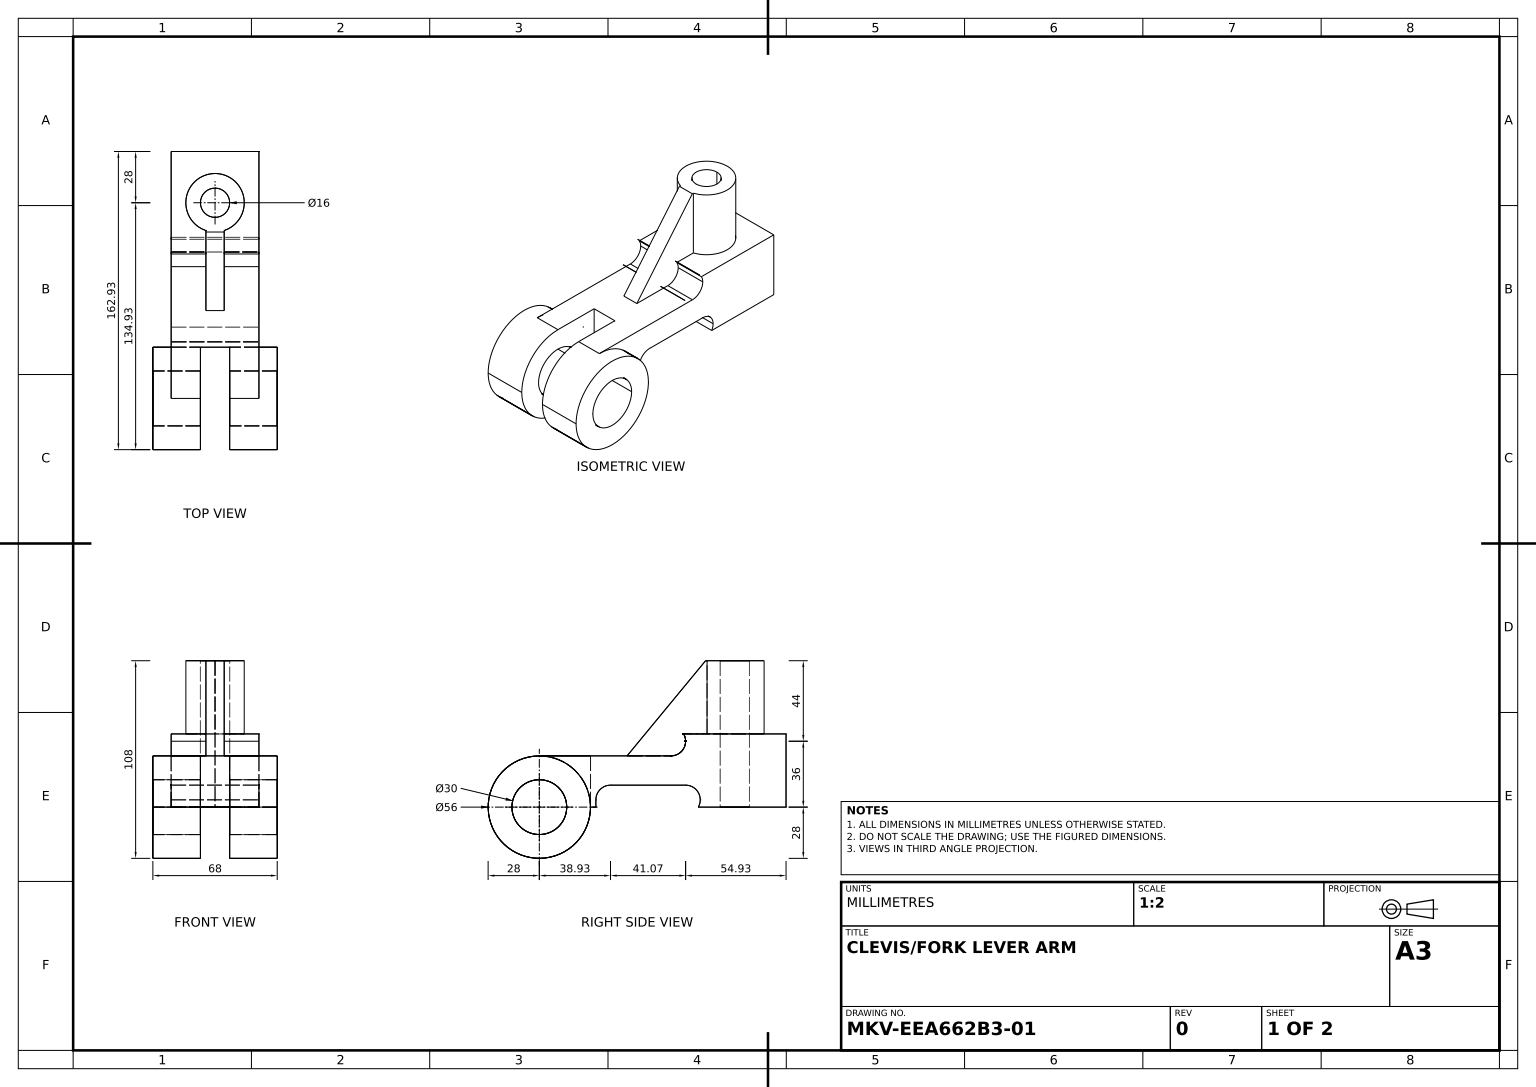
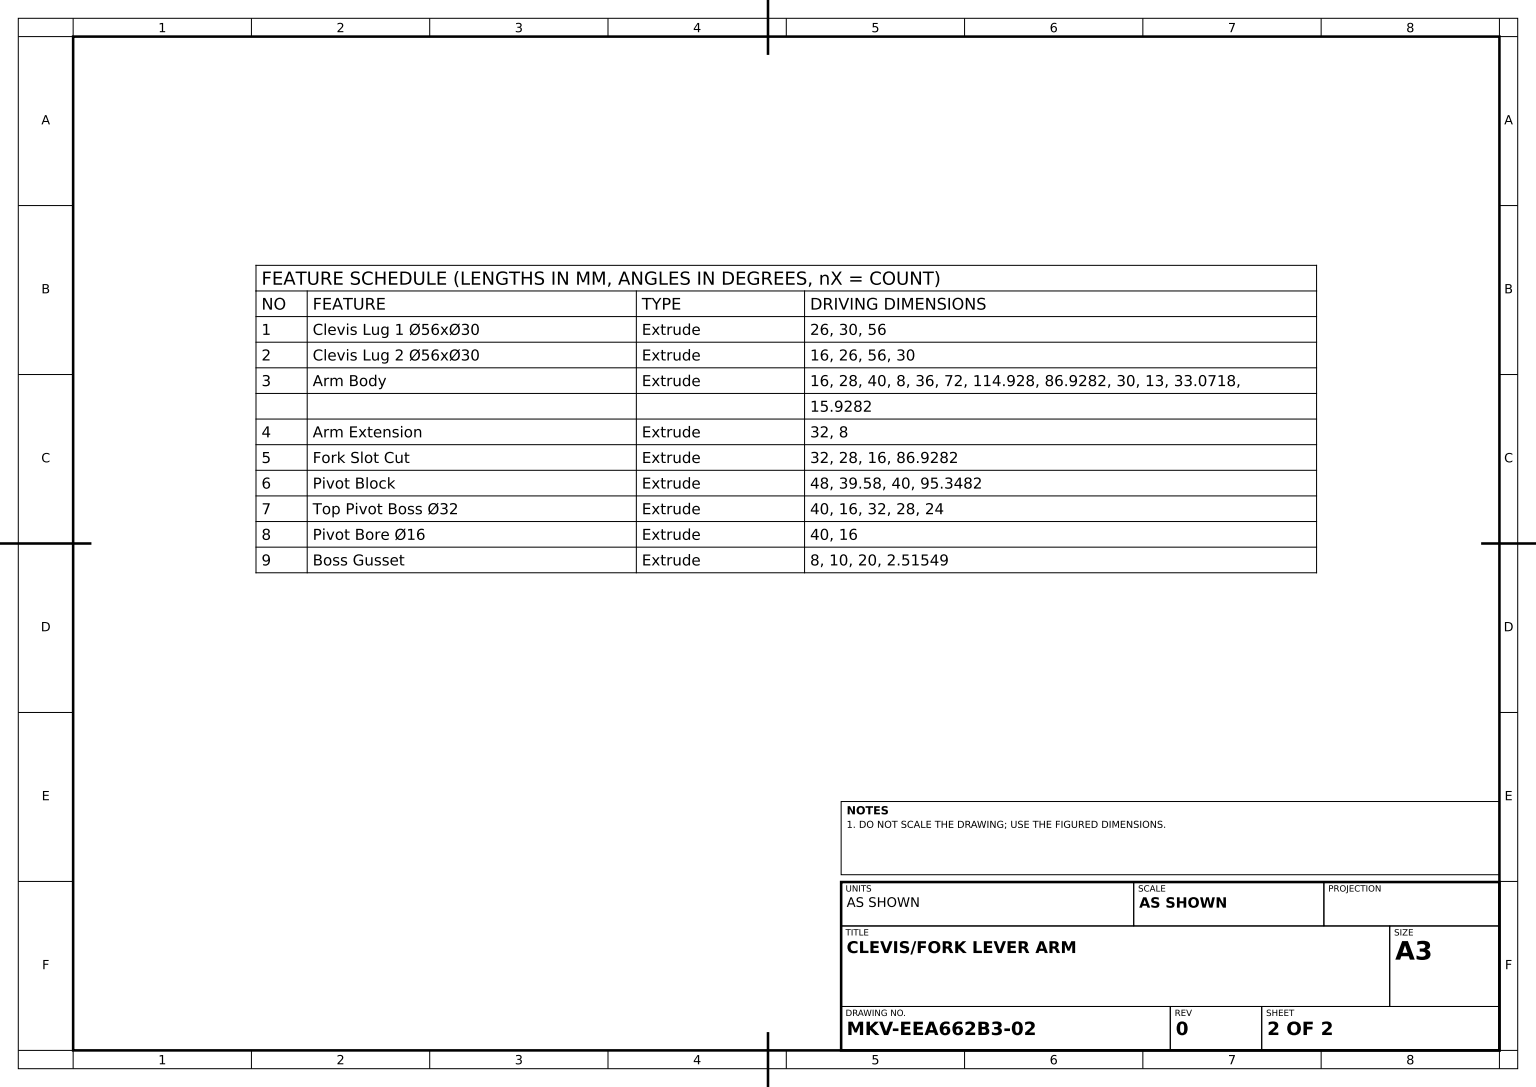
from build123d import *
from build123d.topology import SkipClean

# Parameters (mm, degrees)
CLEVIS_LUG_1_SKETCH_R     = 28
CLEVIS_LUG_1_SKETCH_R_2   = 15
CLEVIS_LUG_1_56X_30_DEPTH = 26
CLEVIS_LUG_2_SKETCH_R     = 28
CLEVIS_LUG_2_SKETCH_R_2   = 15
CLEVIS_LUG_2_56X_30_DEPTH = 26
ARM_START                 = -16
ARM_BODY_DEPTH            = 16
ARM_EXTENSION_DEPTH       = 16
FORK_SLOT_SKETCH_W        = 16
FORK_SLOT_SKETCH_H        = 28
FORK_SLOT_CUT_DEPTH       = 32
PIVOT_BLOCK_SKETCH_W      = 39.579982786
PIVOT_BLOCK_SKETCH_H      = 40
PIVOT_BLOCK_DEPTH         = 48
TOP_PIVOT_BOSS_SKETCH_R   = 16
TOP_PIVOT_BOSS_SKETCH_R_2 = 8
TOP_PIVOT_BOSS_32_DEPTH   = 40
PIVOT_START               = -40
PIVOT_BORE_SKETCH_R       = 8
PIVOT_BORE_16_DEPTH       = 40
BOSS_GUSSET_DEPTH         = 5


with BuildPart() as part:
    # Clevis Lug 1 Sketch → Clevis Lug 1 Ø56xØ30 (new body)
    with BuildSketch(Plane(origin=(0, 0, 0), x_dir=(0, 0, -1), z_dir=(1, 0, 0))):
        with Locations(Location((0, 0, 0), (0, 0, 180))):
            Circle(CLEVIS_LUG_1_SKETCH_R)
        with Locations(Location((0, 0, 0), (0, 0, 180))):
            Circle(CLEVIS_LUG_1_SKETCH_R_2, mode=Mode.SUBTRACT)
    extrude(amount=CLEVIS_LUG_1_56X_30_DEPTH)



with BuildPart() as body_2:
    # Clevis Lug 2 Sketch → Clevis Lug 2 Ø56xØ30 (new body)
    with BuildSketch(Plane(origin=(-16, 0, 0), x_dir=(0, 0, -1), z_dir=(1, 0, 0))):
        with Locations(Location((0, 0, 0), (0, 0, 180))):
            Circle(CLEVIS_LUG_2_SKETCH_R)
        with Locations(Location((0, 0, 0), (0, 0, 180))):
            Circle(CLEVIS_LUG_2_SKETCH_R_2, mode=Mode.SUBTRACT)
    extrude(amount=-CLEVIS_LUG_2_56X_30_DEPTH)

    # Arm Profile Sketch → Arm Body (add)
    with BuildSketch(Plane(origin=(-16, 0, 0), x_dir=(0, 0, -1), z_dir=(1, 0, 0)).offset(ARM_START)):
        with BuildLine():
            Line((72, 28), (0, 28))
            ThreePointArc((0, 28), (19.798989873, 19.798989873), (28, 0))
            Line((28, 0), (30.92820323, 0))
            Line((30.92820323, 0), (30.92820323, 4))
            ThreePointArc((30.92820323, 4), (33.271348981, 9.656854249), (38.92820323, 12))
            Line((38.92820323, 12), (72, 12))
            Line((72, 12), (80, 12))
            ThreePointArc((80, 12), (86.92820323, 8), (86.92820323, 0))
            Line((86.92820323, 0), (114.92820323, 0))
            Line((114.92820323, 0), (114.92820323, 40))
            Line((114.92820323, 40), (78.92820323, 40))
            ThreePointArc((78.92820323, 40), (78.92820323, 32), (72, 28))
        make_face()
    extrude(amount=ARM_BODY_DEPTH)


with BuildPart() as part_1:
    with SkipClean():  # the faces are left unmerged after this step: merging them gives an invalid solid
        add(part.part)

        add(body_2.part)  # Arm Extension merges body 2
        # Arm Extension Sketch → Arm Extension (add, symmetric)
        with BuildSketch(Plane.ZY):
            with BuildLine():
                Line((0, 28), (-72, 28))
                ThreePointArc((-72, 28), (-78.92820323, 32), (-78.92820323, 40))
                Line((-78.92820323, 40), (-114.92820323, 40))
                Line((-114.92820323, 40), (-114.92820323, 0))
                Line((-114.92820323, 0), (-86.92820323, 0))
                ThreePointArc((-86.92820323, 0), (-86.92820323, 8), (-80, 12))
                Line((-80, 12), (-38.92820323, 12))
                ThreePointArc((-38.92820323, 12), (-33.271348981, 9.656854249), (-30.92820323, 4))
                Line((-30.92820323, 4), (-30.92820323, 0))
                Line((-30.92820323, 0), (-15, 0))
                ThreePointArc((-15, 0), (-10.606601718, 10.606601718), (0, 15))
                Line((0, 15), (0, 28))
            make_face()
        extrude(amount=ARM_EXTENSION_DEPTH, both=True)

    # Fork Slot Sketch → Fork Slot Cut (cut)
    with BuildSketch(Plane(origin=(0, 28, 0), x_dir=(1, 0, 0), z_dir=(0, 1, 0))):
        with Locations((-8, 14)):
            Rectangle(FORK_SLOT_SKETCH_W, FORK_SLOT_SKETCH_H)
    extrude(amount=-FORK_SLOT_CUT_DEPTH, mode=Mode.SUBTRACT)

    # Pivot Block Sketch → Pivot Block (add)
    with BuildSketch(Plane(origin=(16, 0, 0), x_dir=(0, 0, -1), z_dir=(1, 0, 0))):
        with Locations((115.138211837, 20)):
            Rectangle(PIVOT_BLOCK_SKETCH_W, PIVOT_BLOCK_SKETCH_H)
    extrude(amount=-PIVOT_BLOCK_DEPTH)

    # Top Pivot Boss Sketch → Top Pivot Boss Ø32 (add)
    with BuildSketch(Plane(origin=(0, 40, 0), x_dir=(1, 0, 0), z_dir=(0, 1, 0))):
        with Locations(Location((-8, 106.92820323, 0), (0, 0, 90))):
            Circle(TOP_PIVOT_BOSS_SKETCH_R)
        with Locations(Location((-8, 106.92820323, 0), (0, 0, 270))):
            Circle(TOP_PIVOT_BOSS_SKETCH_R_2, mode=Mode.SUBTRACT)
    extrude(amount=TOP_PIVOT_BOSS_32_DEPTH)

    # Pivot Bore Sketch → Pivot Bore Ø16 (cut)
    with BuildSketch(Plane(origin=(0, 40, 0), x_dir=(1, 0, 0), z_dir=(0, 1, 0)).offset(PIVOT_START)):
        with Locations(Location((-8, 106.92820323, 0), (0, 0, 270))):
            Circle(PIVOT_BORE_SKETCH_R)
    extrude(amount=PIVOT_BORE_16_DEPTH, mode=Mode.SUBTRACT)

    # Boss Gusset Sketch → Boss Gusset (add, symmetric)
    with BuildSketch(Plane(origin=(-8, 0, 0), x_dir=(0, 0, -1), z_dir=(1, 0, 0))):
        with BuildLine():
            Line((90.92820323, 80), (48, 28))
            Line((48, 28), (72, 28))
            ThreePointArc((72, 28), (78.92820323, 32), (78.92820323, 40))
            Line((78.92820323, 40), (93.443690624, 40))
            Line((93.443690624, 40), (93.443690624, 80))
            Line((93.443690624, 80), (90.92820323, 80))
        make_face()
    extrude(amount=BOSS_GUSSET_DEPTH, both=True)


solid = part_1.part
